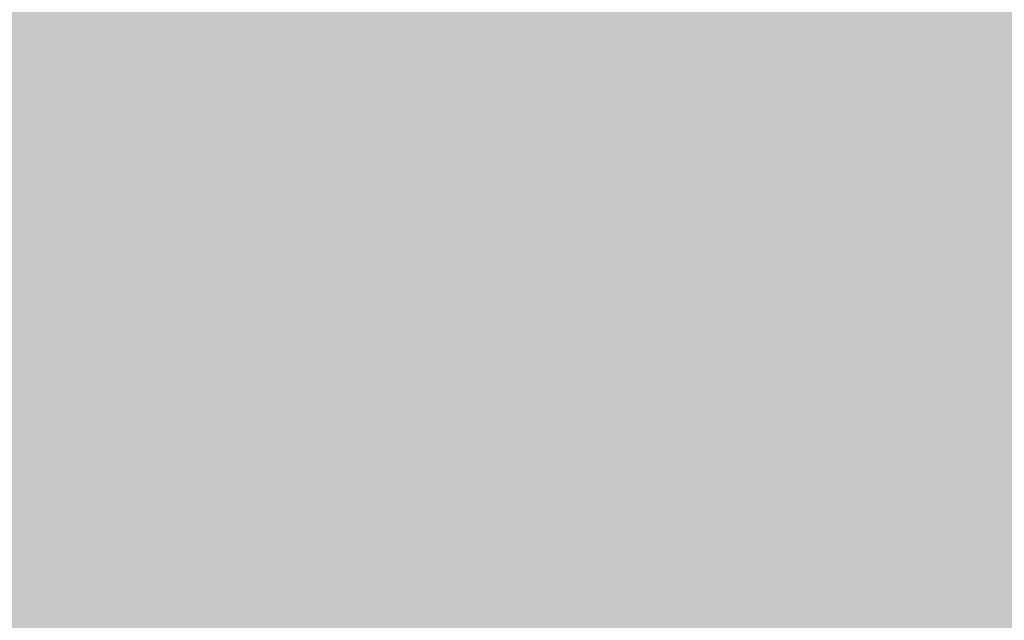
# Model space of a CAD drawing. Units: feet. Extents: x 3168 to 4724, y 827 to 1477.
# Tile 50 of 256: x 3273.072 to 3274.148, y 1098.344 to 1099.001. Entities that reach past the tile are written whole.
import ezdxf

# ---------------------------------------------------------------- set-up
doc = ezdxf.new("R2010")
doc.units = ezdxf.units.FT
doc.layers.add('A-ELEV', color=7, linetype='Continuous', lineweight=35)
doc.layers.add('A-ELEV-PATT', color=8, linetype='Continuous', lineweight=13)

msp = doc.modelspace()

# ---------------------------------------------------------------- hatches: boundary and pattern name
at = {"layer": 'A-ELEV-PATT'}
h = msp.add_hatch(color=256, dxfattribs=at)
h.dxf.hatch_style = 1
edge = h.paths.add_edge_path()
edge.add_ellipse((3552.9058, 979.2201), major_axis=(36.7449, 0), ratio=0.4848485, start_angle=0, end_angle=360)
edge = h.paths.add_edge_path()
edge.add_ellipse((3559.8916, 929.2523), major_axis=(36.7449, 0), ratio=0.4848485, start_angle=0, end_angle=360)
edge = h.paths.add_edge_path()
edge.add_line((3299.3168, 1198.6061), (3479.9167, 1198.6061))
edge.add_line((3479.9167, 1198.6061), (3479.9167, 1209.8686))
edge.add_spline(control_points=[(3479.9167, 1209.8686), (3464.3012, 1209.8686), (3448.6856, 1209.8686), (3410.9491, 1209.8686), (3388.8282, 1209.8686), (3355.6469, 1209.8686), (3344.5864, 1209.8686), (3327.9957, 1209.8686), (3322.4655, 1209.8686), (3314.1702, 1209.8686), (3311.4051, 1209.8686), (3307.2574, 1209.8686), (3305.8748, 1209.8686), (3303.801, 1209.8686), (3303.1097, 1209.8686), (3302.0728, 1209.8686), (3301.7272, 1209.8686), (3301.2087, 1209.8686), (3301.0359, 1209.8686), (3300.7767, 1209.8686), (3300.6903, 1209.8686), (3300.5606, 1209.8686), (3300.5174, 1209.8686), (3300.4526, 1209.8686), (3300.431, 1209.8686), (3300.3986, 1209.8686), (3300.3878, 1209.8686), (3300.3662, 1209.8686), (3300.3457, 1209.8686), (3300.3455, 1209.8686), (3300.3455, 1209.8686), (3300.3433, 1209.8686), (3300.3411, 1209.8686), (3300.3379, 1209.8686), (3300.3368, 1209.8686), (3300.3339, 1209.8686), (3300.3321, 1209.8686), (3300.3255, 1209.8686), (3300.3207, 1209.8686), (3300.3109, 1209.8686), (3300.306, 1209.8686), (3300.2905, 1209.8686), (3300.28, 1209.8686), (3300.2324, 1209.8688), (3300.1953, 1209.869), (3299.9511, 1209.8706), (3299.7448, 1209.8743), (3299.4368, 1209.8833), (3299.3344, 1209.8868), (3299.1811, 1209.8929), (3299.13, 1209.8951), (3298.6522, 1209.9168), (3298.2295, 1209.9457), (3297.6016, 1210.0024), (3297.3934, 1210.0235), (3297.0827, 1210.0583), (3296.9793, 1210.0705), (3296.293, 1210.1549), (3295.7181, 1210.2434), (3294.8687, 1210.3989), (3294.5877, 1210.4545), (3294.1693, 1210.5433), (3294.0304, 1210.5739), (3291.7071, 1211.1012), (3289.6536, 1211.8134), (3285.7763, 1213.564), (3283.9514, 1214.6035), (3280.5122, 1216.9801), (3278.8972, 1218.3176), (3276.3799, 1220.8295), (3275.416, 1221.9177), (3274.0393, 1223.7077), (3273.581, 1224.3495), (3273.1432, 1225.0163)], knot_values=[39.119033, 39.119033, 39.119033, 39.119033, 39.286353, 39.286353, 39.523379, 39.523379, 39.641892, 39.641892, 39.701148, 39.701148, 39.730777, 39.730777, 39.745591, 39.745591, 39.752998, 39.752998, 39.756701, 39.756701, 39.758553, 39.758553, 39.759479, 39.759479, 39.759942, 39.759942, 39.760173, 39.760173, 39.760289, 39.760289, 39.760405, 39.760405, 39.760463, 39.760463, 39.763389, 39.763389, 39.764851, 39.764851, 39.767304, 39.767304, 39.773825, 39.773825, 39.78057, 39.78057, 39.79477, 39.79477, 39.845194, 39.845194, 40.126715, 40.126715, 40.267476, 40.267476, 40.337856, 40.337856, 40.927023, 40.927023, 41.221606, 41.221606, 41.368898, 41.368898, 42.202622, 42.202622, 42.619485, 42.619485, 42.827916, 42.827916, 46.118323, 46.118323, 49.408731, 49.408731, 52.699139, 52.699139, 54.927489, 54.927489, 56.104228, 56.104228, 56.104228, 56.104228], weights=[1, 1, 1, 1, 1, 1, 1, 1, 1, 1, 1, 1, 1, 1, 1, 1, 1, 1, 1, 1, 1, 1, 1, 1, 1, 1, 1, 1, 1, 1, 1, 1, 1, 1, 1, 1, 1, 1, 1, 1, 1, 1, 1, 1, 1, 1, 1, 1, 1, 1, 1, 1, 1, 1, 1, 1, 1, 1, 1, 1, 1, 1, 1, 1, 1, 1, 1, 1, 1, 1, 1, 1, 1, 1], degree=3, periodic=0)
edge.add_line((3273.1432, 1225.0163), (3273.1432, 1099.0163))
edge.add_line((3273.1432, 1099.0163), (3299.3168, 1099.0163))
edge.add_line((3299.3168, 1099.0163), (3299.3168, 1198.6061))
edge = h.paths.add_edge_path()
edge.add_line((3304.7584, 1324.1581), (3479.9167, 1324.1581))
edge.add_line((3479.9167, 1324.1581), (3479.9167, 1335.7146))
edge.add_line((3479.9167, 1335.7146), (3269.1616, 1335.7146))
edge.add_spline(control_points=[(3269.1616, 1335.7146), (3264.0242, 1335.7146), (3258.3641, 1328.9582), (3259.2643, 1323.9003)], knot_values=[0, 0, 0, 0, 15.412191, 15.412191, 15.412191, 15.412191], degree=3, periodic=0)
edge.add_line((3259.2643, 1323.9003), (3265.5168, 1288.7691))
edge.add_line((3265.5168, 1288.7691), (3275.2651, 1261.5456))
edge.add_line((3275.2651, 1261.5456), (3304.7584, 1261.5456))
edge.add_line((3304.7584, 1261.5456), (3304.7584, 1324.1581))
h = msp.add_hatch(color=256, dxfattribs=at)
h.dxf.hatch_style = 1
h.paths.add_polyline_path([(3384.5252, 1099.0163), (3335.0292, 1099.0163), (3299.3168, 1099.0163), (3273.1432, 1099.0163), (3217.5654, 1099.0163), (3168.0693, 827.1163), (3335.0292, 827.1163)])

# ---------------------------------------------------------------- linework, layer by layer
at = {"layer": 'A-ELEV'}
msp.add_open_spline([(3808.5202, 1099.0163), (3808.5202, 1141.4132), (3808.5202, 1183.8102), (3808.5202, 1226.6353), (3808.5202, 1227.0636), (3808.5202, 1227.4918), (3811.4919, 1248.9947), (3814.4635, 1270.4975), (3817.4652, 1292.2176), (3817.4952, 1292.4348), (3817.5253, 1292.652), (3817.5728, 1310.1067), (3817.6203, 1327.5615), (3817.6679, 1345.0163), (3817.6679, 1345.458), (3817.6679, 1345.8996), (3817.6679, 1346.456), (3817.6679, 1346.5708), (3817.6679, 1346.7529), (3817.6679, 1346.8201), (3817.6679, 1346.9349), (3817.6679, 1346.9823), (3817.6679, 1347.0386), (3817.6679, 1347.0474), (3817.6679, 1347.0737), (3817.6679, 1347.0593), (3817.6679, 1347.0615), (3817.6679, 1347.0627), (3817.6679, 1347.066), (3817.6679, 1347.0683), (3817.6679, 1347.075), (3817.6679, 1347.0795), (3817.6678, 1347.0929), (3817.6678, 1347.1019), (3817.6678, 1347.1288), (3817.6677, 1347.1467), (3817.6674, 1347.2004), (3817.6672, 1347.2362), (3817.6661, 1347.3434), (3817.665, 1347.4147), (3817.6608, 1347.6281), (3817.6566, 1347.7697), (3817.64, 1348.1925), (3817.6235, 1348.4716), (3817.5591, 1349.3001), (3817.4961, 1349.8406), (3817.2554, 1351.4242), (3817.0263, 1352.4288), (3816.3069, 1354.8889), (3815.7437, 1356.2687), (3814.464, 1358.8192), (3813.7464, 1359.991), (3812.1958, 1362.1723), (3811.3622, 1363.1821), (3809.5888, 1365.069), (3808.6488, 1365.9461), (3806.6543, 1367.5796), (3805.5997, 1368.3362), (3803.3529, 1369.7223), (3802.1605, 1370.3524), (3799.6008, 1371.4536), (3798.2327, 1371.9255), (3795.2801, 1372.6346), (3793.6931, 1372.8721), (3791.8694, 1372.9265), (3791.7409, 1372.9292), (3791.3534, 1372.9341), (3791.0927, 1372.9329), (3790.3041, 1372.9151), (3789.7695, 1372.8842), (3789.2092, 1372.8302), (3789.1906, 1372.8284), (3789.1349, 1372.8229), (3789.0977, 1372.8191), (3789.0484, 1372.814), (3789.0364, 1372.8127), (3789.0003, 1372.8089), (3788.9761, 1372.8063), (3788.9494, 1372.8034), (3788.9468, 1372.8031), (3788.9426, 1372.8027), (3788.941, 1372.8025), (3788.9386, 1372.8022), (3788.9378, 1372.8021), (3788.9354, 1372.8019), (3788.8675, 1372.7944), (3788.7569, 1372.7822), (3788.7015, 1372.7761), (3788.5355, 1372.7579), (3788.4249, 1372.7457), (3788.0929, 1372.7092), (3787.8715, 1372.6848), (3787.2075, 1372.6118), (3786.7648, 1372.5631), (3785.4368, 1372.417), (3784.5515, 1372.3196), (3781.8954, 1372.0274), (3780.1247, 1371.8327), (3774.8126, 1371.2483), (3771.2713, 1370.8587), (3760.6471, 1369.69), (3753.5643, 1368.9109), (3732.316, 1366.5735), (3718.1504, 1365.0152), (3694.0068, 1362.3593), (3684.0287, 1361.2617), (3674.0506, 1360.1641), (3664.6007, 1360.1641), (3655.1508, 1360.1641), (3626.8011, 1360.1641), (3607.9013, 1360.1641), (3551.2019, 1360.1641), (3513.4023, 1360.1641), (3467.7252, 1360.1641), (3459.8476, 1360.1641), (3436.2149, 1360.1641), (3420.4597, 1360.1641), (3373.1943, 1360.1641), (3341.6839, 1360.1641), (3302.8482, 1360.1641), (3295.5227, 1360.1641), (3286.0383, 1360.1641), (3283.8794, 1360.1641), (3277.4026, 1360.1641), (3273.0848, 1360.1641), (3267.7329, 1360.1641), (3266.6988, 1360.1641), (3263.5965, 1360.1641), (3261.5284, 1360.1641), (3259.2369, 1360.1641), (3259.0137, 1360.1641), (3258.344, 1360.1641), (3257.8975, 1360.1641), (3257.431, 1360.1641), (3257.411, 1360.1641), (3257.3706, 1360.1641), (3257.3755, 1360.1641), (3257.3746, 1360.1641), (3257.3739, 1360.1641), (3257.372, 1360.1641), (3257.3706, 1360.1641), (3257.3667, 1360.1641), (3257.364, 1360.1641), (3257.3561, 1360.1641), (3257.3508, 1360.164), (3257.335, 1360.164), (3257.3244, 1360.164), (3257.2928, 1360.1639), (3257.2717, 1360.1638), (3257.2084, 1360.1634), (3257.1663, 1360.163), (3257.0402, 1360.1614), (3256.9563, 1360.1598), (3256.7055, 1360.1534), (3256.5392, 1360.147), (3256.0436, 1360.1219), (3255.7173, 1360.0971), (3254.7524, 1360.0005), (3254.128, 1359.9065), (3252.1801, 1359.5253), (3250.9416, 1359.144), (3248.6702, 1358.2433), (3247.6357, 1357.7238), (3245.7326, 1356.6035), (3244.8634, 1356.0021), (3243.2531, 1354.7429), (3242.512, 1354.0847), (3240.7511, 1352.3448), (3239.801, 1351.2296), (3238.0878, 1348.8724), (3237.3247, 1347.6304), (3235.9825, 1344.9716), (3235.4022, 1343.5549), (3234.5911, 1340.8155), (3234.3109, 1339.5435), (3233.9765, 1336.8026), (3233.9221, 1335.3309), (3234.1489, 1332.5913), (3234.3495, 1331.3672), (3234.7199, 1329.9994), (3234.7524, 1329.8834), (3234.8536, 1329.5348), (3234.9259, 1329.3017), (3235.0248, 1329.0026), (3235.0469, 1328.9369), (3235.0776, 1328.8472), (3235.0859, 1328.8232), (3235.1109, 1328.7511), (3235.1278, 1328.703), (3235.148, 1328.6462), (3235.1511, 1328.6376), (3235.1561, 1328.6235), (3235.1581, 1328.618), (3235.1602, 1328.612), (3235.1656, 1328.5969), (3235.1801, 1328.5565), (3235.1903, 1328.5281), (3235.2208, 1328.4429), (3235.2411, 1328.3862), (3235.3021, 1328.2159), (3235.3427, 1328.1023), (3235.4647, 1327.7617), (3235.546, 1327.5346), (3235.79, 1326.8534), (3235.9526, 1326.3992), (3236.4405, 1325.0367), (3236.7657, 1324.1284), (3237.7415, 1321.4034), (3238.392, 1319.5868), (3240.3435, 1314.1369), (3241.6445, 1310.5036), (3245.5476, 1299.6037), (3248.1496, 1292.3371), (3255.9557, 1270.5374), (3261.1598, 1256.0042), (3267.3876, 1238.612), (3268.4114, 1235.7529), (3269.5104, 1232.6839), (3269.5856, 1232.4739), (3269.7066, 1232.1359), (3269.7524, 1232.0079), (3269.8273, 1231.7987), (3269.8564, 1231.7176), (3269.9063, 1231.5781), (3269.9272, 1231.5198), (3269.9725, 1231.3934), (3269.9968, 1231.3254), (3270.0265, 1231.2425), (3270.0318, 1231.2277), (3270.0403, 1231.204), (3270.0392, 1231.207), (3270.0394, 1231.2066), (3270.0394, 1231.2064), (3270.0396, 1231.2058), (3270.0398, 1231.2055), (3270.0402, 1231.2043), (3270.0404, 1231.2036), (3270.0413, 1231.2013), (3270.0418, 1231.1998), (3270.0434, 1231.1953), (3270.0445, 1231.1922), (3270.0478, 1231.1832), (3270.0499, 1231.1771), (3270.0564, 1231.159), (3270.0608, 1231.147), (3270.0739, 1231.1108), (3270.0826, 1231.0867), (3270.1089, 1231.0144), (3270.1266, 1230.9663), (3270.1799, 1230.8225), (3270.2159, 1230.7269), (3270.3253, 1230.4415), (3270.4, 1230.2528), (3270.6292, 1229.6914), (3270.7889, 1229.3235), (3271.2865, 1228.2383), (3271.6431, 1227.5398), (3272.7759, 1225.5153), (3273.6142, 1224.2605), (3275.416, 1221.9177), (3276.3799, 1220.8295), (3278.8972, 1218.3176), (3280.5122, 1216.9801), (3283.9514, 1214.6035), (3285.7763, 1213.564), (3289.6536, 1211.8134), (3291.7071, 1211.1012), (3294.0304, 1210.5739), (3294.1693, 1210.5433), (3294.5877, 1210.4545), (3294.8687, 1210.3989), (3295.7181, 1210.2434), (3296.293, 1210.1549), (3296.9793, 1210.0705), (3297.0827, 1210.0583), (3297.3934, 1210.0235), (3297.6016, 1210.0024), (3298.2295, 1209.9457), (3298.6522, 1209.9168), (3299.13, 1209.8951), (3299.1811, 1209.8929), (3299.3344, 1209.8868), (3299.4368, 1209.8833), (3299.7448, 1209.8743), (3299.9511, 1209.8706), (3300.1953, 1209.869), (3300.2324, 1209.8688), (3300.28, 1209.8686), (3300.2905, 1209.8686), (3300.306, 1209.8686), (3300.3109, 1209.8686), (3300.3207, 1209.8686), (3300.3255, 1209.8686), (3300.3321, 1209.8686), (3300.3339, 1209.8686), (3300.3368, 1209.8686), (3300.3379, 1209.8686), (3300.3411, 1209.8686), (3300.3433, 1209.8686), (3300.3455, 1209.8686), (3300.3455, 1209.8686), (3300.3457, 1209.8686), (3300.3662, 1209.8686), (3300.3878, 1209.8686), (3300.3986, 1209.8686), (3300.431, 1209.8686), (3300.4526, 1209.8686), (3300.5174, 1209.8686), (3300.5606, 1209.8686), (3300.6903, 1209.8686), (3300.7767, 1209.8686), (3301.0359, 1209.8686), (3301.2087, 1209.8686), (3301.7272, 1209.8686), (3302.0728, 1209.8686), (3303.1097, 1209.8686), (3303.801, 1209.8686), (3305.8748, 1209.8686), (3307.2574, 1209.8686), (3311.4051, 1209.8686), (3314.1702, 1209.8686), (3322.4655, 1209.8686), (3327.9957, 1209.8686), (3344.5864, 1209.8686), (3355.6469, 1209.8686), (3388.8282, 1209.8686), (3410.9491, 1209.8686), (3477.3119, 1209.8686), (3521.5537, 1209.8686), (3566.8362, 1209.8686), (3567.8769, 1209.8686), (3570.999, 1209.8686), (3573.0804, 1209.8686), (3575.7814, 1209.8686), (3576.4009, 1209.8686), (3577.2958, 1209.8686), (3577.5712, 1209.8686), (3578.3971, 1209.8686), (3578.9478, 1209.8686), (3579.7565, 1209.8686), (3580.0145, 1209.8686), (3580.3427, 1209.8686), (3580.3269, 1209.8686), (3580.3272, 1209.8686), (3580.3273, 1209.8686), (3580.3278, 1209.8686), (3580.3281, 1209.8686), (3580.329, 1209.8686), (3580.3296, 1209.8686), (3580.3314, 1209.8686), (3580.3327, 1209.8686), (3580.3363, 1209.8686), (3580.3388, 1209.8686), (3580.3461, 1209.8686), (3580.351, 1209.8686), (3580.3657, 1209.8685), (3580.3754, 1209.8685), (3580.4048, 1209.8684), (3580.4244, 1209.8684), (3580.4832, 1209.8681), (3580.5224, 1209.8678), (3580.6404, 1209.8666), (3580.7192, 1209.8655), (3580.9563, 1209.8608), (3581.1152, 1209.8561), (3581.5942, 1209.8372), (3581.9164, 1209.8183), (3582.8899, 1209.7424), (3583.548, 1209.6662), (3585.5318, 1209.3606), (3586.8672, 1209.0539), (3589.4715, 1208.2525), (3590.7402, 1207.7579), (3591.9955, 1207.1588), (3592.0578, 1207.1287), (3592.2442, 1207.038), (3592.3677, 1206.9766), (3592.7353, 1206.7904), (3592.9768, 1206.6631), (3593.2445, 1206.5164), (3593.2747, 1206.4998), (3593.3651, 1206.4498), (3593.4251, 1206.4163), (3593.6043, 1206.3153), (3593.7227, 1206.2472), (3593.8572, 1206.1684), (3593.8744, 1206.1583), (3593.9257, 1206.128), (3593.9599, 1206.1078), (3594.0621, 1206.0469), (3594.1298, 1206.0061), (3594.2084, 1205.9582), (3594.2197, 1205.9513), (3594.2534, 1205.9307), (3594.2758, 1205.9169), (3594.343, 1205.8755), (3594.3876, 1205.8479), (3594.4336, 1205.819), (3594.4353, 1205.818), (3594.4402, 1205.8149), (3594.4435, 1205.8129), (3594.4471, 1205.8106), (3594.4475, 1205.8103), (3594.4487, 1205.8096), (3594.4495, 1205.8091), (3594.4504, 1205.8086), (3594.4505, 1205.8085), (3594.4506, 1205.8084), (3594.4674, 1205.7979), (3594.4933, 1205.7817), (3594.5062, 1205.7736), (3594.545, 1205.7492), (3594.5709, 1205.733), (3594.6485, 1205.6844), (3594.7002, 1205.652), (3594.8554, 1205.5547), (3594.9589, 1205.4898), (3595.2694, 1205.2953), (3595.4763, 1205.1656), (3596.0972, 1204.7765), (3596.5111, 1204.5171), (3597.7528, 1203.7388), (3598.5807, 1203.22), (3601.0642, 1201.6636), (3602.7198, 1200.6259), (3607.6868, 1197.513), (3610.9981, 1195.4377), (3620.932, 1189.2119), (3627.5546, 1185.0614), (3647.4225, 1172.6097), (3660.6678, 1164.3086), (3700.4035, 1139.4053), (3726.894, 1122.8031), (3757.2057, 1103.8061), (3761.027, 1101.4112), (3764.8482, 1099.0163), (3745.3283, 1099.0163), (3725.8083, 1099.0163), (3706.2884, 1099.0163), (3706.2884, 1108.4532), (3706.2884, 1117.8902), (3706.2884, 1127.3271), (3710.7508, 1127.3271), (3715.2131, 1127.3271), (3719.6755, 1127.3271)], degree=3, knots=[0, 0, 0, 0, 0.982037, 0.982037, 0.991957, 0.991957, 0.991957, 1.966522, 1.966522, 1.976367, 1.976367, 1.976367, 2.976367, 2.976367, 2.976367, 3.00169, 3.00169, 3.008272, 3.008272, 3.012129, 3.012129, 3.014851, 3.014851, 3.015353, 3.015353, 3.016359, 3.016359, 3.017365, 3.017365, 3.019376, 3.019376, 3.023398, 3.023398, 3.031442, 3.031442, 3.047531, 3.047531, 3.079708, 3.079708, 3.144063, 3.144063, 3.272772, 3.272772, 3.53019, 3.53019, 4.045026, 4.045026, 5.074698, 5.074698, 6.700878, 6.700878, 8.327058, 8.327058, 9.953238, 9.953238, 11.579418, 11.579418, 13.205598, 13.205598, 14.831778, 14.831778, 16.457958, 16.457958, 18.084138, 18.084138, 18.206872, 18.206872, 18.45234, 18.45234, 18.943275, 18.943275, 18.960093, 18.960093, 18.993729, 18.993729, 19.00461, 19.00461, 19.026374, 19.026374, 19.028737, 19.028737, 19.03018, 19.03018, 19.030897, 19.030897, 19.032332, 19.032332, 19.033766, 19.033766, 19.036636, 19.036636, 19.042374, 19.042374, 19.053851, 19.053851, 19.076805, 19.076805, 19.122714, 19.122714, 19.21453, 19.21453, 19.398163, 19.398163, 19.765429, 19.765429, 20.024128, 20.024128, 20.024128, 20.092031, 20.092031, 20.227836, 20.227836, 20.499446, 20.499446, 20.556051, 20.556051, 20.66926, 20.66926, 20.895678, 20.895678, 20.948316, 20.948316, 20.963829, 20.963829, 20.994855, 20.994855, 21.002285, 21.002285, 21.017146, 21.017146, 21.01875, 21.01875, 21.021959, 21.021959, 21.022102, 21.022102, 21.022249, 21.022249, 21.022708, 21.022708, 21.023627, 21.023627, 21.025464, 21.025464, 21.029138, 21.029138, 21.036486, 21.036486, 21.051183, 21.051183, 21.080575, 21.080575, 21.139361, 21.139361, 21.256932, 21.256932, 21.492073, 21.492073, 21.962356, 21.962356, 23.01002, 23.01002, 24.057684, 24.057684, 25.105348, 25.105348, 26.153011, 26.153011, 27.776787, 27.776787, 29.400562, 29.400562, 31.024337, 31.024337, 32.278801, 32.278801, 33.533265, 33.533265, 34.467568, 34.467568, 34.553971, 34.553971, 34.726776, 34.726776, 34.775309, 34.775309, 34.793079, 34.793079, 34.82862, 34.82862, 34.834979, 34.834979, 34.839039, 34.839039, 34.839411, 34.839411, 34.840285, 34.840285, 34.842034, 34.842034, 34.845531, 34.845531, 34.852525, 34.852525, 34.866512, 34.866512, 34.894488, 34.894488, 34.950439, 34.950439, 35.062342, 35.062342, 35.286147, 35.286147, 35.733758, 35.733758, 35.821815, 35.821815, 35.828283, 35.828283, 35.832225, 35.832225, 35.834724, 35.834724, 35.836521, 35.836521, 35.838617, 35.838617, 35.839073, 35.839073, 35.839345, 35.839345, 35.839617, 35.839617, 35.840161, 35.840161, 35.841249, 35.841249, 35.843425, 35.843425, 35.847778, 35.847778, 35.856482, 35.856482, 35.873891, 35.873891, 35.908709, 35.908709, 35.978345, 35.978345, 36.117617, 36.117617, 36.396161, 36.396161, 36.953248, 36.953248, 38.067423, 38.067423, 40.295772, 40.295772, 42.524122, 42.524122, 45.81453, 45.81453, 49.104937, 49.104937, 52.395345, 52.395345, 52.603776, 52.603776, 53.020639, 53.020639, 53.854363, 53.854363, 54.001655, 54.001655, 54.296238, 54.296238, 54.885405, 54.885405, 54.955785, 54.955785, 55.096546, 55.096546, 55.378067, 55.378067, 55.42849, 55.42849, 55.442691, 55.442691, 55.449436, 55.449436, 55.455957, 55.455957, 55.458409, 55.458409, 55.459872, 55.459872, 55.462798, 55.462798, 55.462856, 55.462856, 55.462972, 55.462972, 55.463088, 55.463088, 55.463319, 55.463319, 55.463782, 55.463782, 55.464708, 55.464708, 55.46656, 55.46656, 55.470263, 55.470263, 55.47767, 55.47767, 55.492484, 55.492484, 55.522112, 55.522112, 55.581369, 55.581369, 55.699882, 55.699882, 55.936907, 55.936907, 56.410959, 56.410959, 56.42211, 56.42211, 56.444413, 56.444413, 56.451051, 56.451051, 56.454001, 56.454001, 56.459901, 56.459901, 56.462666, 56.462666, 56.463418, 56.463418, 56.464171, 56.464171, 56.465675, 56.465675, 56.468684, 56.468684, 56.474702, 56.474702, 56.486738, 56.486738, 56.51081, 56.51081, 56.558955, 56.558955, 56.655243, 56.655243, 56.847821, 56.847821, 57.232975, 57.232975, 58.003284, 58.003284, 59.543901, 59.543901, 62.625137, 62.625137, 68.787607, 68.787607, 74.950078, 74.950078, 75.27336, 75.27336, 75.919923, 75.919923, 77.213051, 77.213051, 77.377769, 77.377769, 77.707206, 77.707206, 78.366079, 78.366079, 78.462532, 78.462532, 78.655436, 78.655436, 79.041245, 79.041245, 79.105735, 79.105735, 79.234714, 79.234714, 79.492672, 79.492672, 79.502197, 79.502197, 79.521249, 79.521249, 79.523534, 79.523534, 79.528103, 79.528103, 79.528682, 79.528682, 79.528885, 79.528885, 79.529089, 79.529089, 79.529495, 79.529495, 79.530308, 79.530308, 79.531935, 79.531935, 79.535187, 79.535187, 79.541693, 79.541693, 79.554704, 79.554704, 79.580725, 79.580725, 79.632769, 79.632769, 79.736856, 79.736856, 79.94503, 79.94503, 80.361377, 80.361377, 80.421435, 80.421435, 80.421435, 81.421435, 81.421435, 81.421435, 82.421435, 82.421435, 82.421435, 83.421435, 83.421435, 83.421435, 83.421435], dxfattribs=at)

doc.saveas('drawing.dxf')
